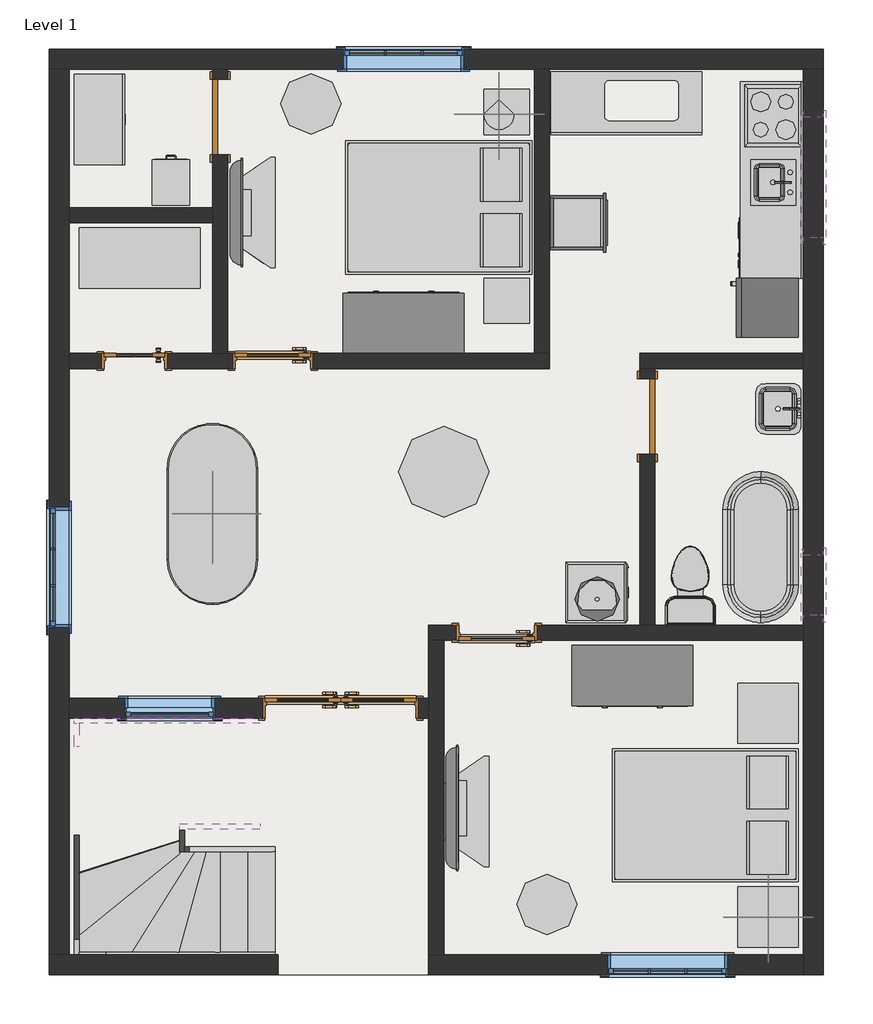
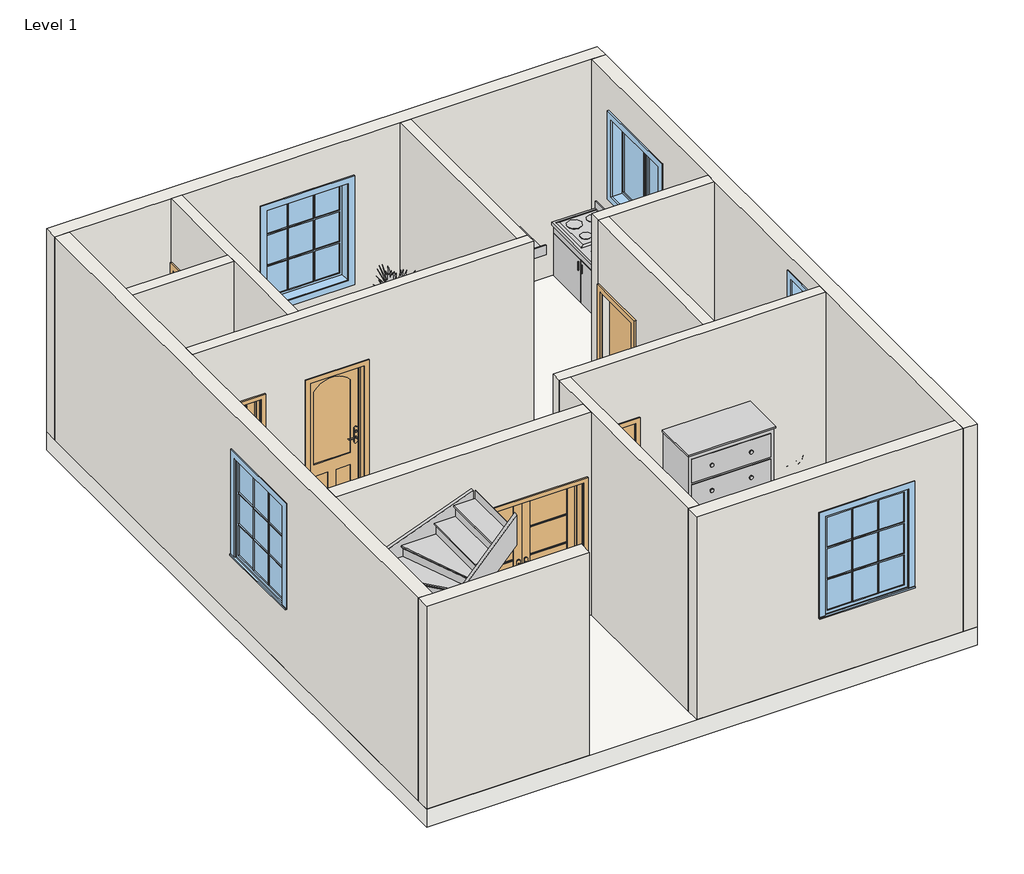
# One storey, incomplete: 22 furniture elements, 14 walls, 8 members, 6 doors, 6 windows, 5 flow terminals, 5 proxies, 3 geographic elements, 2 other elements.
"""IFC4 building model written with IfcOpenShell, lengths in millimetres."""

from ifc_helpers import new_model, si_unit, frame, origin, origin_with_axes, place, context, project, spatial, polyline, outline, extrude, faceted_brep, transform, mapped, element, save
from components import proxy_a6faaae8, proxy_45b28599, kitchenette_medium_kitchenette_medium_844211aa, proxy_8b8c2dc4, proxy_c523a7b7, door_4b146b56, door_14b9be53, door_b03bd389, door_6d64ae12, door_255cab33, door_059fdd7e, flow_terminal_871c2e40, flow_terminal_d49f872f, flow_terminal_62a433f7, toilet_domestic_3d_toilet_domestic_3d_f7549cf7, toilet_domestic_3d_toilet_domestic_3d_183bbd19, flow_terminal_b374fae2, furniture_6a014568, furniture_c8abb964, furniture_552c1472, furniture_c6510c7c, furniture_c9930e7d, furniture_2babcf72, furniture_9fa109b2, furniture_e1dba61b, furniture_7a3aaa4f, furniture_fdf74506, tv_stand_tv_stand_6ce107e5, furniture_2c34a4f9, furniture_905aceb5, furniture_f0d1c541, furniture_097b63cf, furniture_5bc9ed15, furniture_51091a24, rpc_plant_tropical_55f6ff97, rpc_plant_tropical_agave_1_5_93a2a214, stair_flight_22c751ce, window_cfa1ffdd, window_0862ab64, window_31198920, window_e41d21a6

model = new_model("IFC4")

# Units and contexts
model_context = context("Model", 3, world=origin())
ifc_project = project(units=[si_unit("LENGTHUNIT", "METRE", prefix="MILLI")], contexts=[model_context])

# Site, building, storey
site = spatial("IfcSite", under=ifc_project)
building = spatial("IfcBuilding", under=site)
storey = spatial("IfcBuildingStorey", under=building, Name="Level 1", Elevation=0.0)

# Proxies
placement = place(None, origin())
proxy_shape = proxy_a6faaae8(model_context)
element("IfcBuildingElementProxy", 1, Name="Cook Top-4 Unit2 : 22\" x 20\"", ObjectType="Cook Top-4 Unit2 : 22\" x 20\"", at=placement, inside=storey, context=model_context, shape_type="MappedRepresentation", body=[
    mapped(proxy_shape, transform((-2789.082173, 12884.8549175, 0.0), x_axis=(0.0, -1.0000000000000002, 0.0), y_axis=(1.0000000000000002, 0.0, 0.0), z_axis=(0.0, 0.0, 1.0))),
])
proxy_2_shape = proxy_45b28599(model_context)
element("IfcBuildingElementProxy", 2, Name="Dishwasher : 24\" x 24\" x 34\"", ObjectType="Dishwasher : 24\" x 24\" x 34\"", at=placement, inside=storey, context=model_context, shape_type="MappedRepresentation", body=[
    mapped(proxy_2_shape, transform((-3080.9317378, 11933.672386, 0.0), x_axis=(0.0, -1.0000000000000002, 0.0), y_axis=(1.0000000000000002, 0.0, 0.0), z_axis=(0.0, 0.0, 1.0))),
])
kitchenette_medium_kitchenette_medium_shape = kitchenette_medium_kitchenette_medium_844211aa(model_context)
element("IfcBuildingElementProxy", 3, Name="Kitchenette - Medium : Kitchenette - Medium", ObjectType="Kitchenette - Medium : Kitchenette - Medium", at=placement, inside=storey, context=model_context, shape_type="MappedRepresentation", body=[
    mapped(kitchenette_medium_kitchenette_medium_shape, transform((-2484.282173, 12560.6926225, 0.0), x_axis=(0.0, -1.0000000000000002, 0.0), y_axis=(1.0000000000000002, 0.0, 0.0), z_axis=(0.0, 0.0, 1.0))),
])
proxy_3_shape = proxy_8b8c2dc4(model_context)
element("IfcBuildingElementProxy", 4, Name="Oven Double-Built-in : 21 1/2\" x 39 1/4\" x 21\"", ObjectType="Oven Double-Built-in : 21 1/2\" x 39 1/4\" x 21\"", at=placement, inside=storey, context=model_context, shape_type="MappedRepresentation", body=[
    mapped(proxy_3_shape, transform((-4629.2163141, 11840.5298448, 0.0), x_axis=(0.0, 1.0000000000000009, 0.0), y_axis=(-1.0000000000000009, 0.0, 0.0), z_axis=(0.0, 0.0, 1.0))),
])
proxy_4_shape = proxy_c523a7b7(model_context)
element("IfcBuildingElementProxy", 5, Name="Refrigerator : 24\" x 25\" LH", ObjectType="Refrigerator : 24\" x 25\" LH", at=placement, inside=storey, context=model_context, shape_type="MappedRepresentation", body=[
    mapped(proxy_4_shape, transform((-2834.7311445, 10948.1049175, 0.0), x_axis=(0.0, -1.0000000000000002, 0.0), y_axis=(1.0000000000000002, 0.0, 0.0), z_axis=(0.0, 0.0, 1.0))),
])

# Doors
door_shape = door_4b146b56(model_context)
element("IfcDoor", 6, ObjectType="30\" x 80\"", at=placement, inside=storey, context=model_context, shape_type="MappedRepresentation", body=[
    mapped(door_shape, transform((-5583.082173, 7661.9799175, 0.0), x_axis=(1.0, 0.0, 0.0), y_axis=(0.0, 1.0, 0.0), z_axis=(0.0, 0.0, 1.0))),
])
door_2_shape = door_14b9be53(model_context)
element("IfcDoor", 7, ObjectType="30\" x 80\"", at=placement, inside=storey, context=model_context, shape_type="MappedRepresentation", body=[
    mapped(door_2_shape, transform((-7843.682173, 10411.5299175, 0.0), x_axis=(1.0, 0.0, 0.0), y_axis=(0.0, 1.0, 0.0), z_axis=(0.0, 0.0, 1.0))),
])
door_3_shape = door_b03bd389(model_context)
element("IfcDoor", 8, ObjectType="Door-Exterior-Double-Full Glass-Wood_Clad : 60\" x 80\"", at=placement, inside=storey, context=model_context, shape_type="MappedRepresentation", body=[
    mapped(door_3_shape, transform((-7157.882173, 6906.3299175, 0.0), x_axis=(1.0, 0.0, 0.0), y_axis=(0.0, 1.0, 0.0), z_axis=(0.0, 0.0, 1.0))),
])
door_4_shape = door_6d64ae12(model_context)
element("IfcDoor", 9, ObjectType="Door-Interior-Single-Full Glass-Wood : 24\" x 80\"", at=placement, inside=storey, context=model_context, shape_type="MappedRepresentation", body=[
    mapped(door_4_shape, transform((-9240.682173, 10411.5299175, 0.0), x_axis=(-1.0, 0.0, 0.0), y_axis=(0.0, -1.0, 0.0), z_axis=(0.0, 0.0, 1.0))),
])
door_5_shape = door_255cab33(model_context)
element("IfcDoor", 10, ObjectType="Single-Flush : 30\" x 80\"", at=placement, inside=storey, context=model_context, shape_type="MappedRepresentation", body=[
    mapped(door_5_shape, transform((-4059.082173, 9849.5549175, 0.0), x_axis=(0.0, 1.0, 0.0), y_axis=(-1.0, 0.0, 0.0), z_axis=(0.0, 0.0, 1.0))),
])
door_6_shape = door_059fdd7e(model_context)
element("IfcDoor", 11, ObjectType="Single-Flush : 30\" x 80\"", at=placement, inside=storey, context=model_context, shape_type="MappedRepresentation", body=[
    mapped(door_6_shape, transform((-8377.082173, 12872.1549175, 0.0), x_axis=(0.0, 1.0, 0.0), y_axis=(-1.0, 0.0, 0.0), z_axis=(0.0, 0.0, 1.0))),
])

# Flow terminals
flow_terminal_shape = flow_terminal_871c2e40(model_context)
element("IfcFlowTerminal", 12, ObjectType="Sink Kitchen-Island : 18\" x 18\"", at=placement, inside=storey, context=model_context, shape_type="MappedRepresentation", body=[
    mapped(flow_terminal_shape, transform((-2791.4275741, 12227.4441581, -14.4), x_axis=(0.0, -1.0000000000000002, 0.0), y_axis=(1.0000000000000002, 0.0, 0.0), z_axis=(0.0, 0.0, 1.0))),
])
flow_terminal_2_shape = flow_terminal_d49f872f(model_context)
element("IfcFlowTerminal", 13, ObjectType="Sink Vanity-Round : 19\" x 19\"", at=placement, inside=storey, context=model_context, shape_type="MappedRepresentation", body=[
    mapped(flow_terminal_2_shape, transform((-4470.4304324, 8089.8607114, 457.2), x_axis=(-1.0, 0.0, 0.0), y_axis=(0.0, -1.0, 0.0), z_axis=(0.0, 0.0, 1.0))),
])
flow_terminal_3_shape = flow_terminal_62a433f7(model_context)
element("IfcFlowTerminal", 14, ObjectType="Sink Vanity-Square : 20\" x 18\"", at=placement, inside=storey, context=model_context, shape_type="MappedRepresentation", body=[
    mapped(flow_terminal_3_shape, transform((-2689.8275741, 9941.4441581, 0.0), x_axis=(0.0, -1.0000000000000004, 0.0), y_axis=(1.0000000000000004, 0.0, 0.0), z_axis=(0.0, 0.0, 1.0))),
])
toilet_domestic_3d_toilet_domestic_3d_shape = toilet_domestic_3d_toilet_domestic_3d_f7549cf7(model_context)
toilet_domestic_3d_toilet_domestic_3d_2_shape = toilet_domestic_3d_toilet_domestic_3d_183bbd19(model_context)
element("IfcFlowTerminal", 15, ObjectType="Toilet-Domestic-3D : Toilet-Domestic-3D", at=placement, inside=storey, context=model_context, shape_type="MappedRepresentation", body=[
    mapped(toilet_domestic_3d_toilet_domestic_3d_shape, transform((-3627.282173, 8236.0509449, 0.0), x_axis=(-1.0000000000000004, 0.0, 0.0), y_axis=(0.0, -1.0000000000000004, 0.0), z_axis=(0.0, 0.0, 1.0))),
    mapped(toilet_domestic_3d_toilet_domestic_3d_2_shape, transform((-3627.282173, 8236.0509449, 0.0), x_axis=(-1.0000000000000004, 0.0, 0.0), y_axis=(0.0, -1.0000000000000004, 0.0), z_axis=(0.0, 0.0, 1.0))),
])
flow_terminal_4_shape = flow_terminal_b374fae2(model_context)
element("IfcFlowTerminal", 16, ObjectType="Tub-Free Standing-3D : 30\" x 60\"", at=placement, inside=storey, context=model_context, shape_type="MappedRepresentation", body=[
    mapped(flow_terminal_4_shape, transform((-2916.082173, 8528.7549175, 0.0), x_axis=(-1.0000000000000004, 0.0, 0.0), y_axis=(0.0, -1.0000000000000004, 0.0), z_axis=(0.0, 0.0, 1.0))),
])

# Furniture
furniture_shape = furniture_6a014568(model_context)
element("IfcFurniture", 17, ObjectType="24\"", at=placement, inside=storey, context=model_context, shape_type="MappedRepresentation", body=[
    mapped(furniture_shape, transform((-4884.582173, 8052.8172126, 0.0), x_axis=(0.0, 1.0, 0.0), y_axis=(-1.0, 0.0, 0.0), z_axis=(0.0, 0.0, 1.0))),
])
furniture_2_shape = furniture_c8abb964(model_context)
element("IfcFurniture", 18, ObjectType="Bed-Box : Double 53\" x 74\"", at=placement, inside=storey, context=model_context, shape_type="MappedRepresentation", body=[
    mapped(furniture_2_shape, transform((-3240.4526648, 6162.8073766, 0.0), x_axis=(0.0, -0.9999999999999998, 0.0), y_axis=(0.9999999999999998, 0.0, 0.0), z_axis=(0.0, 0.0, 1.0))),
])
element("IfcFurniture", 19, ObjectType="Bed-Box : Double 53\" x 74\"", at=placement, inside=storey, context=model_context, shape_type="MappedRepresentation", body=[
    mapped(furniture_2_shape, transform((-5932.8526648, 12296.9073766, 0.0), x_axis=(0.0, -1.0000000000000002, 0.0), y_axis=(1.0000000000000002, 0.0, 0.0), z_axis=(0.0, 0.0, 1.0))),
])
furniture_3_shape = furniture_552c1472(model_context)
element("IfcFurniture", 20, ObjectType="Cabinet-File 3 Drawer.0001 : 15\" x 18\"", at=placement, inside=storey, context=model_context, shape_type="MappedRepresentation", body=[
    mapped(furniture_3_shape, transform((-9000.27862, 12069.6206174, 0.0), x_axis=(-1.0000000000000004, 0.0, 0.0), y_axis=(0.0, -1.0000000000000004, 0.0), z_axis=(0.0, 0.0, 1.0))),
])
furniture_4_shape = furniture_c6510c7c(model_context)
element("IfcFurniture", 21, ObjectType="Counter Top w Sink Hole : 24\" Depth", at=placement, inside=storey, context=model_context, shape_type="MappedRepresentation", body=[
    mapped(furniture_4_shape, transform((-2484.282173, 12027.2926225, -14.4), x_axis=(0.0, -1.0000000000000002, 0.0), y_axis=(1.0000000000000002, 0.0, 0.0), z_axis=(0.0, 0.0, 1.0))),
])
furniture_5_shape = furniture_c9930e7d(model_context)
element("IfcFurniture", 22, ObjectType="Counter Top w Sink Hole : 24\" Depth", at=placement, inside=storey, context=model_context, shape_type="MappedRepresentation", body=[
    mapped(furniture_5_shape, transform((-4708.7182214, 12694.3549175, 0.0), x_axis=(-1.0, 0.0, 0.0), y_axis=(0.0, -1.0, 0.0), z_axis=(0.0, 0.0, 1.0))),
])
furniture_6_shape = furniture_2babcf72(model_context)
element("IfcFurniture", 23, ObjectType="Dresser : 48\" x 60\" x 24\"", at=placement, inside=storey, context=model_context, shape_type="MappedRepresentation", body=[
    mapped(furniture_6_shape, transform((-6792.0754328, 10426.1919634, 0.0), x_axis=(-1.0000000000000004, 0.0, 0.0), y_axis=(0.0, -1.0000000000000004, 0.0), z_axis=(0.0, 0.0, 1.0))),
])
furniture_7_shape = furniture_9fa109b2(model_context)
element("IfcFurniture", 24, ObjectType="Dresser : 48\" x 72\" x 24\"", at=placement, inside=storey, context=model_context, shape_type="MappedRepresentation", body=[
    mapped(furniture_7_shape, transform((-3941.830498, 7596.5178716, 0.0), x_axis=(1.0, 0.0, 0.0), y_axis=(0.0, 1.0, 0.0), z_axis=(0.0, 0.0, 1.0))),
])
furniture_8_shape = furniture_e1dba61b(model_context)
element("IfcFurniture", 25, ObjectType="Storage Pedestal : 20\" x 36\" x 36\"", at=placement, inside=storey, context=model_context, shape_type="MappedRepresentation", body=[
    mapped(furniture_8_shape, transform((-10530.6005491, 13026.7774315, 0.0), x_axis=(0.0, 1.000000000000001, 0.0), y_axis=(-1.000000000000001, 0.0, 0.0), z_axis=(0.0, 0.0, 1.0))),
])
furniture_9_shape = furniture_7a3aaa4f(model_context)
element("IfcFurniture", 26, ObjectType="TV - Flat Screen : 42\"", at=placement, inside=storey, context=model_context, shape_type="MappedRepresentation", body=[
    mapped(furniture_9_shape, transform((-8216.9435494, 11910.8994317, 914.4), x_axis=(0.0, 1.0000000000000002, 0.0), y_axis=(-1.0000000000000002, 0.0, 0.0), z_axis=(0.0, 0.0, 1.0))),
])
furniture_10_shape = furniture_fdf74506(model_context)
element("IfcFurniture", 27, ObjectType="TV - Flat Screen : 50\"", at=placement, inside=storey, context=model_context, shape_type="MappedRepresentation", body=[
    mapped(furniture_10_shape, transform((-6037.9435494, 5898.1815114, 914.4), x_axis=(0.0, 1.0, 0.0), y_axis=(-1.0, 0.0, 0.0), z_axis=(0.0, 0.0, 1.0))),
])
tv_stand_tv_stand_shape = tv_stand_tv_stand_6ce107e5(model_context)
element("IfcFurniture", 28, ObjectType="TV Stand : TV Stand", at=placement, inside=storey, context=model_context, shape_type="MappedRepresentation", body=[
    mapped(tv_stand_tv_stand_shape, transform((-6116.482173, 5736.5669155, 0.0), x_axis=(0.0, 1.0000000000000002, 0.0), y_axis=(-1.0000000000000002, 0.0, 0.0), z_axis=(0.0, 0.0, 1.0))),
])
element("IfcFurniture", 29, ObjectType="TV Stand : TV Stand", at=placement, inside=storey, context=model_context, shape_type="MappedRepresentation", body=[
    mapped(tv_stand_tv_stand_shape, transform((-8275.482173, 11781.7669155, 0.0), x_axis=(0.0, 1.0000000000000002, 0.0), y_axis=(-1.0000000000000002, 0.0, 0.0), z_axis=(0.0, 0.0, 1.0))),
])
furniture_11_shape = furniture_2c34a4f9(model_context)
element("IfcFurniture", 30, ObjectType="Table-Dining Oval : 36\" x 72\"", at=placement, inside=storey, context=model_context, shape_type="MappedRepresentation", body=[
    mapped(furniture_11_shape, transform((-8811.3805337, 9266.7122138, 0.0), x_axis=(0.0, 1.0, 0.0), y_axis=(-1.0, 0.0, 0.0), z_axis=(0.0, 0.0, 1.0))),
])
furniture_12_shape = furniture_905aceb5(model_context)
element("IfcFurniture", 31, ObjectType="Table-Dining Round w Chairs : 36\" Diameter", at=placement, inside=storey, context=model_context, shape_type="MappedRepresentation", body=[
    mapped(furniture_12_shape, transform((-6220.1641402, 9475.6336061, 0.0), x_axis=(1.0, 0.0, 0.0), y_axis=(0.0, 1.0, 0.0), z_axis=(0.0, 0.0, 1.0))),
])
furniture_13_shape = furniture_f0d1c541(model_context)
element("IfcFurniture", 32, ObjectType="Table-Ellipse : 72\" x 36\"", at=placement, inside=storey, context=model_context, shape_type="MappedRepresentation", body=[
    mapped(furniture_13_shape, transform((-5075.082173, 4921.9549175, 0.0), x_axis=(-1.0000000000000004, 0.0, 0.0), y_axis=(0.0, -1.0000000000000004, 0.0), z_axis=(0.0, 0.0, 1.0))),
])
element("IfcFurniture", 33, ObjectType="Table-Ellipse : 72\" x 36\"", at=placement, inside=storey, context=model_context, shape_type="MappedRepresentation", body=[
    mapped(furniture_13_shape, transform((-7459.1574537, 13005.1582156, 0.0), x_axis=(0.0, 1.000000000000001, 0.0), y_axis=(-1.000000000000001, 0.0, 0.0), z_axis=(0.0, 0.0, 1.0))),
])
furniture_14_shape = furniture_097b63cf(model_context)
element("IfcFurniture", 34, ObjectType="Table-Night Stand : 18\" x 18\" x 24\"", at=placement, inside=storey, context=model_context, shape_type="MappedRepresentation", body=[
    mapped(furniture_14_shape, transform((-5713.8158033, 10789.3549175, 0.0), x_axis=(1.0, 0.0, 0.0), y_axis=(0.0, 1.0, 0.0), z_axis=(0.0, 0.0, 1.0))),
])
element("IfcFurniture", 35, ObjectType="Table-Night Stand : 18\" x 18\" x 24\"", at=placement, inside=storey, context=model_context, shape_type="MappedRepresentation", body=[
    mapped(furniture_14_shape, transform((-5713.8158033, 12694.3549175, 0.0), x_axis=(1.0, 0.0, 0.0), y_axis=(0.0, 1.0, 0.0), z_axis=(0.0, 0.0, 1.0))),
])
furniture_15_shape = furniture_5bc9ed15(model_context)
element("IfcFurniture", 36, ObjectType="Table-Night Stand : 24\" x 24\" x 30\"", at=placement, inside=storey, context=model_context, shape_type="MappedRepresentation", body=[
    mapped(furniture_15_shape, transform((-3148.4158033, 4490.1549175, 0.0), x_axis=(1.0, 0.0, 0.0), y_axis=(0.0, 1.0, 0.0), z_axis=(0.0, 0.0, 1.0))),
])
element("IfcFurniture", 37, ObjectType="Table-Night Stand : 24\" x 24\" x 30\"", at=placement, inside=storey, context=model_context, shape_type="MappedRepresentation", body=[
    mapped(furniture_15_shape, transform((-3148.4158033, 6547.5549175, 0.0), x_axis=(1.0, 0.0, 0.0), y_axis=(0.0, 1.0, 0.0), z_axis=(0.0, 0.0, 1.0))),
])
furniture_16_shape = furniture_51091a24(model_context)
element("IfcFurniture", 38, ObjectType="Table-Rectangular : 72\" x 30\"", at=placement, inside=storey, context=model_context, shape_type="MappedRepresentation", body=[
    mapped(furniture_16_shape, transform((-9189.882173, 11449.7549175, 0.0), x_axis=(1.0, 0.0, 0.0), y_axis=(0.0, 1.0, 0.0), z_axis=(0.0, 0.0, 1.0))),
])

# Geographic elements
rpc_plant_tropical_shape = rpc_plant_tropical_55f6ff97(model_context)
element("IfcGeographicElement", 39, ObjectType="RPC Plant - Tropical", at=placement, inside=storey, context=model_context, shape_type="MappedRepresentation", body=[
    mapped(rpc_plant_tropical_shape, transform((-8453.282173, 8864.8925416, 609.6), x_axis=(1.0, 0.0, 0.0), y_axis=(0.0, 1.0, 0.0), z_axis=(0.0, 0.0, 1.0))),
])
rpc_plant_tropical_agave_1_5_shape = rpc_plant_tropical_agave_1_5_93a2a214(model_context)
element("IfcGeographicElement", 40, ObjectType="RPC Plant - Tropical : Agave - 1.5'", at=placement, inside=storey, context=model_context, shape_type="MappedRepresentation", body=[
    mapped(rpc_plant_tropical_agave_1_5_shape, transform((-5557.682173, 12897.5549175, 762.0), x_axis=(1.0, 0.0, 0.0), y_axis=(0.0, 1.0, 0.0), z_axis=(0.0, 0.0, 1.0))),
])
element("IfcGeographicElement", 41, ObjectType="RPC Plant - Tropical : Agave - 1.5'", at=placement, inside=storey, context=model_context, shape_type="MappedRepresentation", body=[
    mapped(rpc_plant_tropical_agave_1_5_shape, transform((-2839.882173, 4794.9549175, 762.0), x_axis=(1.0, 0.0, 0.0), y_axis=(0.0, 1.0, 0.0), z_axis=(0.0, 0.0, 1.0))),
])

# Members
element("IfcMember", 42, ObjectType="Stringer - 2\" Width", at=placement, inside=storey, context=model_context, shape_type="SweptSolid", body=[
    extrude(outline(polyline([(83.5564967, -7818.2848745), (415.8418245, -7818.2848745), (1159.7595923, -9531.8106114), (827.4742644, -9531.8106114), (83.5564967, -7818.2848745)])), frame((0.0, 4388.5549175, 0.0), z_axis=(0.0, 1.0, 0.0), x_axis=(0.0, 0.0, 1.0)), (0.0, 0.0, 1.0), 50.8),
])
element("IfcMember", 43, ObjectType="Stringer - 2\" Width", at=placement, inside=storey, context=model_context, shape_type="SweptSolid", body=[
    extrude(outline(polyline([(-9531.8106114, 4439.3549175), (-9531.8106114, 4388.5549175), (-9799.482173, 4388.5549175), (-9799.482173, 4439.3549175), (-9531.8106114, 4439.3549175)])), frame((0.0, 0.0, 827.4742644), z_axis=(0.0, 0.0, 1.0), x_axis=(1.0, 0.0, 0.0)), (0.0, 0.0, 1.0), 332.2853278),
])
element("IfcMember", 44, ObjectType="Stringer - 2\" Width", at=placement, inside=storey, context=model_context, shape_type="SweptSolid", body=[
    extrude(outline(polyline([(4388.5549175, 854.9595923), (4388.5549175, 1143.7120466), (6514.0452981, 1815.1471627), (6514.0452981, 1482.8618349), (4526.3622821, 854.9595923), (4388.5549175, 854.9595923)])), frame((-9850.282173, 0.0, 0.0), z_axis=(1.0, 0.0, 0.0), x_axis=(0.0, 1.0, 0.0)), (0.0, 0.0, 1.0), 50.8),
])
element("IfcMember", 45, ObjectType="Stringer - 2\" Width", at=placement, inside=storey, context=model_context, shape_type="SweptSolid", body=[
    extrude(outline(polyline([(-9799.482173, 6514.0452981), (-9850.282173, 6514.0452981), (-9850.282173, 6750.7549175), (-9799.482173, 6750.7549175), (-9799.482173, 6514.0452981)])), frame((0.0, 0.0, 1489.2492928), z_axis=(0.0, 0.0, 1.0), x_axis=(1.0, 0.0, 0.0)), (0.0, 0.0, 1.0), 319.6465141),
])
element("IfcMember", 46, ObjectType="Stringer - 2\" Width", at=placement, inside=storey, context=model_context, shape_type="SweptSolid", body=[
    extrude(outline(polyline([(1789.6968643, -9850.282173), (1504.0958069, -9850.282173), (1504.0958069, -9760.1986078), (2179.5047781, -7973.0806206), (2499.1512922, -7973.0806206), (1789.6968643, -9850.282173)])), frame((0.0, 6750.7549175, 0.0), z_axis=(0.0, 1.0, 0.0), x_axis=(0.0, 0.0, 1.0)), (0.0, 0.0, 1.0), 50.8),
])
element("IfcMember", 47, ObjectType="Stringer - 2\" Width", at=placement, inside=storey, context=model_context, shape_type="SweptSolid", body=[
    extrude(outline(polyline([(0.0, -7818.2848745), (314.6605696, -7818.2848745), (1250.7228943, -8732.682173), (814.5341975, -8732.682173), (0.0, -7937.000251), (0.0, -7818.2848745)])), frame((0.0, 5455.3549175, 0.0), z_axis=(0.0, 1.0, 0.0), x_axis=(0.0, 0.0, 1.0)), (0.0, 0.0, 1.0), 50.8),
])
element("IfcMember", 48, ObjectType="Stringer - 2\" Width", at=placement, inside=storey, context=model_context, shape_type="SweptSolid", body=[
    extrude(outline(polyline([(5455.3549175, 866.5378136), (5455.3549175, 1470.7613416), (5640.3509671, 1890.0468689), (5683.9549175, 1890.0468689), (5683.9549175, 1233.8039522), (5521.9107248, 866.5378136), (5455.3549175, 866.5378136)])), frame((-8783.482173, 0.0, 0.0), z_axis=(1.0, 0.0, 0.0), x_axis=(0.0, 1.0, 0.0)), (0.0, 0.0, 1.0), 50.8),
])
element("IfcMember", 49, ObjectType="Stringer - 2\" Width", at=placement, inside=storey, context=model_context, shape_type="SweptSolid", body=[
    extrude(outline(polyline([(1890.0468689, -8783.482173), (1436.8245927, -8783.482173), (2328.6417632, -7973.0806206), (2781.8640394, -7973.0806206), (1890.0468689, -8783.482173)])), frame((0.0, 5683.9549175, 0.0), z_axis=(0.0, 1.0, 0.0), x_axis=(0.0, 0.0, 1.0)), (0.0, 0.0, 1.0), 50.8),
])

# Slab
element("IfcSlab", 50, ObjectType="Wood Joist 10\" - Ceramic Tile", at=placement, inside=storey, context=model_context, shape_type="SweptSolid", body=[
    extrude(outline(polyline([(-2281.082173, 13557.9549175), (-2281.082173, 4210.7549175), (-10104.282173, 4210.7549175), (-10104.282173, 13557.9549175), (-2281.082173, 13557.9549175)])), frame((0.0, 0.0, -273.05), z_axis=(0.0, 0.0, 1.0), x_axis=(1.0, 0.0, 0.0)), (0.0, 0.0, 1.0), 273.05),
])

# Stair flight
stair_flight_shape = stair_flight_22c751ce(model_context)
element("IfcStairFlight", 51, ObjectType="2\" Tread 1\" Nosing 1/4\" Riser", at=placement, inside=storey, context=model_context, shape_type="MappedRepresentation", body=[
    mapped(stair_flight_shape, transform((0.0, 0.0, 0.0), x_axis=(1.0, 0.0, 0.0), y_axis=(0.0, 1.0, 0.0), z_axis=(0.0, 0.0, 1.0))),
])

# Walls
element("IfcWall", 52, ObjectType="Generic - 8\"", at=placement, inside=storey, context=model_context, shape_type="Brep", body=[
    faceted_brep([(-10104.282173, 13354.7549175, 0.0), (-9901.082173, 13354.7549175, 0.0), (-8453.282173, 13354.7549175, 0.0), (-8300.882173, 13354.7549175, 0.0), (-5202.082173, 13354.7549175, 0.0), (-5049.682173, 13354.7549175, 0.0), (-2484.282173, 13354.7549175, 0.0), (-2281.082173, 13354.7549175, 0.0), (-2281.082173, 13354.7549175, 3048.0), (-2484.282173, 13354.7549175, 3048.0), (-5049.682173, 13354.7549175, 3048.0), (-5202.082173, 13354.7549175, 3048.0), (-8300.882173, 13354.7549175, 3048.0), (-8453.282173, 13354.7549175, 3048.0), (-9901.082173, 13354.7549175, 3048.0), (-10104.282173, 13354.7549175, 3048.0), (-5913.282173, 13354.7549175, 2438.4), (-5913.282173, 13354.7549175, 914.4), (-7132.482173, 13354.7549175, 914.4), (-7132.482173, 13354.7549175, 2438.4), (-10104.282173, 13557.9549175, 0.0), (-10104.282173, 13557.9549175, 3048.0), (-2281.082173, 13557.9549175, 3048.0), (-2281.082173, 13557.9549175, 0.0), (-5913.282173, 13557.9549175, 2438.4), (-7132.482173, 13557.9549175, 2438.4), (-7132.482173, 13557.9549175, 914.4), (-5913.282173, 13557.9549175, 914.4)], [[[0, 1, 2, 3, 4, 5, 6, 7, 8, 9, 10, 11, 12, 13, 14, 15], [16, 17, 18, 19]], [[20, 21, 22, 23], [24, 25, 26, 27]], [[7, 6, 5, 4, 3, 2, 1, 0, 20, 23]], [[8, 7, 23, 22]], [[0, 15, 21, 20]], [[15, 14, 13, 12, 11, 10, 9, 8, 22, 21]], [[17, 16, 24, 27]], [[18, 17, 27, 26]], [[19, 18, 26, 25]], [[16, 19, 25, 24]]]),
])
element("IfcWall", 53, ObjectType="Generic - 8\"", at=placement, inside=storey, context=model_context, shape_type="Brep", body=[
    faceted_brep([(-2484.282173, 13354.7549175, 0.0), (-2484.282173, 10484.5549175, 0.0), (-2484.282173, 10332.1549175, 0.0), (-2484.282173, 7741.3549175, 0.0), (-2484.282173, 7588.9549175, 0.0), (-2484.282173, 4413.9549175, 0.0), (-2484.282173, 4210.7549175, 0.0), (-2484.282173, 4210.7549175, 3048.0), (-2484.282173, 4413.9549175, 3048.0), (-2484.282173, 7588.9549175, 3048.0), (-2484.282173, 7741.3549175, 3048.0), (-2484.282173, 10332.1549175, 3048.0), (-2484.282173, 10484.5549175, 3048.0), (-2484.282173, 13354.7549175, 3048.0), (-2484.282173, 11652.9549175, 2489.2), (-2484.282173, 11652.9549175, 1270.0), (-2484.282173, 12872.1549175, 1270.0), (-2484.282173, 12872.1549175, 2489.2), (-2484.282173, 7842.9549175, 2768.6), (-2484.282173, 7842.9549175, 2159.0), (-2484.282173, 8452.5549175, 2159.0), (-2484.282173, 8452.5549175, 2768.6), (-2281.082173, 13354.7549175, 0.0), (-2281.082173, 13354.7549175, 3048.0), (-2281.082173, 4210.7549175, 3048.0), (-2281.082173, 4210.7549175, 0.0), (-2281.082173, 11652.9549175, 2489.2), (-2281.082173, 12872.1549175, 2489.2), (-2281.082173, 12872.1549175, 1270.0), (-2281.082173, 11652.9549175, 1270.0), (-2281.082173, 7842.9549175, 2768.6), (-2281.082173, 8452.5549175, 2768.6), (-2281.082173, 8452.5549175, 2159.0), (-2281.082173, 7842.9549175, 2159.0)], [[[0, 1, 2, 3, 4, 5, 6, 7, 8, 9, 10, 11, 12, 13], [14, 15, 16, 17], [18, 19, 20, 21]], [[22, 23, 24, 25], [26, 27, 28, 29], [30, 31, 32, 33]], [[6, 5, 4, 3, 2, 1, 0, 22, 25]], [[0, 13, 23, 22]], [[7, 6, 25, 24]], [[13, 12, 11, 10, 9, 8, 7, 24, 23]], [[15, 14, 26, 29]], [[16, 15, 29, 28]], [[17, 16, 28, 27]], [[14, 17, 27, 26]], [[19, 18, 30, 33]], [[20, 19, 33, 32]], [[21, 20, 32, 31]], [[18, 21, 31, 30]]]),
])
element("IfcWall", 54, ObjectType="Generic - 8\"", at=placement, inside=storey, context=model_context, shape_type="Brep", body=[
    faceted_brep([(-2484.282173, 4413.9549175, 0.0), (-6116.482173, 4413.9549175, 0.0), (-6268.882173, 4413.9549175, 0.0), (-6268.882173, 4413.9549175, 3048.0), (-6116.482173, 4413.9549175, 3048.0), (-2484.282173, 4413.9549175, 3048.0), (-4465.482173, 4413.9549175, 2438.4), (-4465.482173, 4413.9549175, 914.4), (-3246.282173, 4413.9549175, 914.4), (-3246.282173, 4413.9549175, 2438.4), (-2484.282173, 4210.7549175, 0.0), (-2484.282173, 4210.7549175, 3048.0), (-6268.882173, 4210.7549175, 3048.0), (-6268.882173, 4210.7549175, 0.0), (-4465.482173, 4210.7549175, 2438.4), (-3246.282173, 4210.7549175, 2438.4), (-3246.282173, 4210.7549175, 914.4), (-4465.482173, 4210.7549175, 914.4)], [[[0, 1, 2, 3, 4, 5], [6, 7, 8, 9]], [[10, 11, 12, 13], [14, 15, 16, 17]], [[2, 1, 0, 10, 13]], [[0, 5, 11, 10]], [[3, 2, 13, 12]], [[5, 4, 3, 12, 11]], [[7, 6, 14, 17]], [[8, 7, 17, 16]], [[9, 8, 16, 15]], [[6, 9, 15, 14]]]),
])
element("IfcWall", 55, ObjectType="Generic - 8\"", at=placement, inside=storey, context=model_context, shape_type="Brep", body=[
    faceted_brep([(-9901.082173, 4413.9549175, 0.0), (-9901.082173, 6801.5549175, 0.0), (-9901.082173, 7004.7549175, 0.0), (-9901.082173, 10332.1549175, 0.0), (-9901.082173, 10484.5549175, 0.0), (-9901.082173, 11805.3549175, 0.0), (-9901.082173, 11957.7549175, 0.0), (-9901.082173, 13354.7549175, 0.0), (-9901.082173, 13354.7549175, 3048.0), (-9901.082173, 11957.7549175, 3048.0), (-9901.082173, 11805.3549175, 3048.0), (-9901.082173, 10484.5549175, 3048.0), (-9901.082173, 10332.1549175, 3048.0), (-9901.082173, 7004.7549175, 3048.0), (-9901.082173, 6801.5549175, 3048.0), (-9901.082173, 4413.9549175, 3048.0), (-9901.082173, 8935.1549175, 2438.4), (-9901.082173, 8935.1549175, 914.4), (-9901.082173, 7715.9549175, 914.4), (-9901.082173, 7715.9549175, 2438.4), (-10104.282173, 4413.9549175, 0.0), (-10104.282173, 4413.9549175, 3048.0), (-10104.282173, 13354.7549175, 3048.0), (-10104.282173, 13354.7549175, 0.0), (-10104.282173, 8935.1549175, 2438.4), (-10104.282173, 7715.9549175, 2438.4), (-10104.282173, 7715.9549175, 914.4), (-10104.282173, 8935.1549175, 914.4)], [[[0, 1, 2, 3, 4, 5, 6, 7, 8, 9, 10, 11, 12, 13, 14, 15], [16, 17, 18, 19]], [[20, 21, 22, 23], [24, 25, 26, 27]], [[7, 6, 5, 4, 3, 2, 1, 0, 20, 23]], [[8, 7, 23, 22]], [[0, 15, 21, 20]], [[15, 14, 13, 12, 11, 10, 9, 8, 22, 21]], [[17, 16, 24, 27]], [[18, 17, 27, 26]], [[19, 18, 26, 25]], [[16, 19, 25, 24]]]),
])
element("IfcWall", 56, ObjectType="Generic - 8\"", at=placement, inside=storey, context=model_context, shape_type="SweptSolid", body=[
    extrude(outline(polyline([(3048.0, -9901.082173), (0.0, -9901.082173), (0.0, -7945.282173), (2057.4, -7945.282173), (2057.4, -6370.482173), (0.0, -6370.482173), (0.0, -6268.882173), (3048.0, -6268.882173), (3048.0, -9901.082173)]), holes=[polyline([(1778.0, -9342.282173), (1778.0, -8427.882173), (558.8, -8427.882173), (558.8, -9342.282173), (1778.0, -9342.282173)])]), frame((0.0, 6801.5549175, 0.0), z_axis=(0.0, 1.0, 0.0), x_axis=(0.0, 0.0, 1.0)), (0.0, 0.0, 1.0), 203.2),
])
element("IfcWall", 57, ObjectType="Generic - 8\"", at=placement, inside=storey, context=model_context, shape_type="Brep", body=[
    faceted_brep([(-7792.882173, 4413.9549175, 0.0), (-9901.082173, 4413.9549175, 0.0), (-10104.282173, 4413.9549175, 0.0), (-10104.282173, 4413.9549175, 3048.0), (-9901.082173, 4413.9549175, 3048.0), (-7792.882173, 4413.9549175, 3048.0), (-7792.882173, 4210.7549175, 0.0), (-7792.882173, 4210.7549175, 3048.0), (-10104.282173, 4210.7549175, 3048.0), (-10104.282173, 4210.7549175, 0.0)], [[[0, 1, 2, 3, 4, 5]], [[6, 7, 8, 9]], [[2, 1, 0, 6, 9]], [[0, 5, 7, 6]], [[3, 2, 9, 8]], [[5, 4, 3, 8, 7]]]),
])
element("IfcWall", 58, ObjectType="INNER WALL", at=placement, inside=storey, context=model_context, shape_type="Brep", body=[
    faceted_brep([(-2484.282173, 10484.5549175, 0.0), (-4135.282173, 10484.5549175, 0.0), (-4135.282173, 10484.5549175, 3048.0), (-2484.282173, 10484.5549175, 3048.0), (-2484.282173, 10332.1549175, 0.0), (-2484.282173, 10332.1549175, 3048.0), (-3982.882173, 10332.1549175, 3048.0), (-4135.282173, 10332.1549175, 3048.0), (-4135.282173, 10332.1549175, 0.0), (-3982.882173, 10332.1549175, 0.0)], [[[0, 1, 2, 3]], [[4, 5, 6, 7, 8, 9]], [[1, 0, 4, 9, 8]], [[0, 3, 5, 4]], [[2, 1, 8, 7]], [[3, 2, 7, 6, 5]]]),
])
element("IfcWall", 59, ObjectType="INNER WALL", at=placement, inside=storey, context=model_context, shape_type="SweptSolid", body=[
    extrude(outline(polyline([(-5202.082173, 10484.5549175), (-5202.082173, 13354.7549175), (-5049.682173, 13354.7549175), (-5049.682173, 10484.5549175), (-5202.082173, 10484.5549175)])), origin_with_axes(), (0.0, 0.0, 1.0), 3048.0),
])
element("IfcWall", 60, ObjectType="INNER WALL", at=placement, inside=storey, context=model_context, shape_type="Brep", body=[
    faceted_brep([(-8300.882173, 13253.1549175, 2032.0), (-8300.882173, 13253.1549175, 0.0), (-8300.882173, 13354.7549175, 0.0), (-8300.882173, 13354.7549175, 3048.0), (-8300.882173, 10484.5549175, 3048.0), (-8300.882173, 10484.5549175, 0.0), (-8300.882173, 12491.1549175, 0.0), (-8300.882173, 12491.1549175, 2032.0), (-8453.282173, 13354.7549175, 0.0), (-8453.282173, 13253.1549175, 0.0), (-8453.282173, 13253.1549175, 2032.0), (-8453.282173, 12491.1549175, 2032.0), (-8453.282173, 12491.1549175, 0.0), (-8453.282173, 11957.7549175, 0.0), (-8453.282173, 11805.3549175, 0.0), (-8453.282173, 10484.5549175, 0.0), (-8453.282173, 10484.5549175, 3048.0), (-8453.282173, 11805.3549175, 3048.0), (-8453.282173, 11957.7549175, 3048.0), (-8453.282173, 13354.7549175, 3048.0)], [[[0, 1, 2, 3, 4, 5, 6, 7]], [[8, 9, 10, 11, 12, 13, 14, 15, 16, 17, 18, 19]], [[6, 5, 15, 14, 13, 12]], [[2, 1, 9, 8]], [[3, 2, 8, 19]], [[5, 4, 16, 15]], [[10, 9, 1, 0]], [[11, 10, 0, 7]], [[12, 11, 7, 6]], [[4, 3, 19, 18, 17, 16]]]),
])
element("IfcWall", 61, ObjectType="INNER WALL", at=placement, inside=storey, context=model_context, shape_type="Brep", body=[
    faceted_brep([(-2484.282173, 7741.3549175, 3048.0), (-2484.282173, 7741.3549175, 0.0), (-3982.882173, 7741.3549175, 0.0), (-4135.282173, 7741.3549175, 0.0), (-5176.682173, 7741.3549175, 0.0), (-5176.682173, 7741.3549175, 2057.4), (-5989.482173, 7741.3549175, 2057.4), (-5989.482173, 7741.3549175, 0.0), (-6268.882173, 7741.3549175, 0.0), (-6268.882173, 7741.3549175, 3048.0), (-4135.282173, 7741.3549175, 3048.0), (-3982.882173, 7741.3549175, 3048.0), (-2484.282173, 7588.9549175, 0.0), (-2484.282173, 7588.9549175, 3048.0), (-6116.482173, 7588.9549175, 3048.0), (-6268.882173, 7588.9549175, 3048.0), (-6268.882173, 7588.9549175, 0.0), (-6116.482173, 7588.9549175, 0.0), (-5989.482173, 7588.9549175, 0.0), (-5989.482173, 7588.9549175, 2057.4), (-5176.682173, 7588.9549175, 2057.4), (-5176.682173, 7588.9549175, 0.0)], [[[0, 1, 2, 3, 4, 5, 6, 7, 8, 9, 10, 11]], [[12, 13, 14, 15, 16, 17, 18, 19, 20, 21]], [[1, 12, 21, 4, 3, 2]], [[16, 8, 7, 18, 17]], [[1, 0, 13, 12]], [[9, 8, 16, 15]], [[20, 5, 4, 21]], [[5, 20, 19, 6]], [[6, 19, 18, 7]], [[0, 11, 10, 9, 15, 14, 13]]]),
])
element("IfcWall", 62, ObjectType="INNER WALL", at=placement, inside=storey, context=model_context, shape_type="SweptSolid", body=[
    extrude(outline(polyline([(10332.1549175, 0.0), (10230.5549175, 0.0), (10230.5549175, 2032.0), (9468.5549175, 2032.0), (9468.5549175, 0.0), (7741.3549175, 0.0), (7741.3549175, 3048.0), (10332.1549175, 3048.0), (10332.1549175, 0.0)])), frame((-4135.282173, 0.0, 0.0), z_axis=(1.0, 0.0, 0.0), x_axis=(0.0, 1.0, 0.0)), (0.0, 0.0, 1.0), 152.4),
])
element("IfcWall", 63, ObjectType="INNER WALL", at=placement, inside=storey, context=model_context, shape_type="Brep", body=[
    faceted_brep([(-6268.882173, 7588.9549175, 0.0), (-6268.882173, 7004.7549175, 0.0), (-6268.882173, 6801.5549175, 0.0), (-6268.882173, 4413.9549175, 0.0), (-6268.882173, 4413.9549175, 3048.0), (-6268.882173, 6801.5549175, 3048.0), (-6268.882173, 7004.7549175, 3048.0), (-6268.882173, 7588.9549175, 3048.0), (-6116.482173, 7588.9549175, 0.0), (-6116.482173, 7588.9549175, 3048.0), (-6116.482173, 4413.9549175, 3048.0), (-6116.482173, 4413.9549175, 0.0)], [[[0, 1, 2, 3, 4, 5, 6, 7]], [[8, 9, 10, 11]], [[3, 2, 1, 0, 8, 11]], [[4, 3, 11, 10]], [[0, 7, 9, 8]], [[7, 6, 5, 4, 10, 9]]]),
])
element("IfcWall", 64, ObjectType="INNER WALL", at=placement, inside=storey, context=model_context, shape_type="SweptSolid", body=[
    extrude(outline(polyline([(-9901.082173, 11957.7549175), (-8453.282173, 11957.7549175), (-8453.282173, 11805.3549175), (-9901.082173, 11805.3549175), (-9901.082173, 11957.7549175)])), origin_with_axes(), (0.0, 0.0, 1.0), 3048.0),
])
element("IfcWall", 65, ObjectType="INNER WALL", at=placement, inside=storey, context=model_context, shape_type="Brep", body=[
    faceted_brep([(-5049.682173, 10484.5549175, 3048.0), (-5049.682173, 10484.5549175, 0.0), (-5202.082173, 10484.5549175, 0.0), (-7437.282173, 10484.5549175, 0.0), (-7437.282173, 10484.5549175, 2057.4), (-8250.082173, 10484.5549175, 2057.4), (-8250.082173, 10484.5549175, 0.0), (-8300.882173, 10484.5549175, 0.0), (-8453.282173, 10484.5549175, 0.0), (-8910.482173, 10484.5549175, 0.0), (-8910.482173, 10484.5549175, 2057.4), (-9570.882173, 10484.5549175, 2057.4), (-9570.882173, 10484.5549175, 0.0), (-9901.082173, 10484.5549175, 0.0), (-9901.082173, 10484.5549175, 3048.0), (-8453.282173, 10484.5549175, 3048.0), (-8300.882173, 10484.5549175, 3048.0), (-5202.082173, 10484.5549175, 3048.0), (-5049.682173, 10332.1549175, 0.0), (-5049.682173, 10332.1549175, 3048.0), (-9901.082173, 10332.1549175, 3048.0), (-9901.082173, 10332.1549175, 0.0), (-9570.882173, 10332.1549175, 0.0), (-9570.882173, 10332.1549175, 2057.4), (-8910.482173, 10332.1549175, 2057.4), (-8910.482173, 10332.1549175, 0.0), (-8250.082173, 10332.1549175, 0.0), (-8250.082173, 10332.1549175, 2057.4), (-7437.282173, 10332.1549175, 2057.4), (-7437.282173, 10332.1549175, 0.0)], [[[0, 1, 2, 3, 4, 5, 6, 7, 8, 9, 10, 11, 12, 13, 14, 15, 16, 17]], [[18, 19, 20, 21, 22, 23, 24, 25, 26, 27, 28, 29]], [[1, 18, 29, 3, 2]], [[21, 13, 12, 22]], [[6, 26, 25, 9, 8, 7]], [[1, 0, 19, 18]], [[14, 13, 21, 20]], [[28, 4, 3, 29]], [[4, 28, 27, 5]], [[5, 27, 26, 6]], [[11, 23, 22, 12]], [[23, 11, 10, 24]], [[24, 10, 9, 25]], [[0, 17, 16, 15, 14, 20, 19]]]),
])

# Windows
window_shape = window_cfa1ffdd(model_context)
element("IfcWindow", 66, ObjectType="Casement 3x3 with Trim : 48\" x 60\"", at=placement, inside=storey, context=model_context, shape_type="MappedRepresentation", body=[
    mapped(window_shape, transform((-3855.882173, 4312.3549175, 304.8), x_axis=(-1.0, 0.0, 0.0), y_axis=(0.0, -1.0, 0.0), z_axis=(0.0, 0.0, 1.0))),
])
element("IfcWindow", 67, ObjectType="Casement 3x3 with Trim : 48\" x 60\"", at=placement, inside=storey, context=model_context, shape_type="MappedRepresentation", body=[
    mapped(window_shape, transform((-10002.682173, 8325.5549175, 304.8), x_axis=(0.0, 1.0, 0.0), y_axis=(-1.0, 0.0, 0.0), z_axis=(0.0, 0.0, 1.0))),
])
element("IfcWindow", 68, ObjectType="Casement 3x3 with Trim : 48\" x 60\"", at=placement, inside=storey, context=model_context, shape_type="MappedRepresentation", body=[
    mapped(window_shape, transform((-6522.882173, 13456.3549175, 304.8), x_axis=(1.0, 0.0, 0.0), y_axis=(0.0, 1.0, 0.0), z_axis=(0.0, 0.0, 1.0))),
])
window_2_shape = window_0862ab64(model_context)
element("IfcWindow", 69, ObjectType="Casement Dbl with Trim : 48\" x 48\"", at=placement, inside=storey, context=model_context, shape_type="MappedRepresentation", body=[
    mapped(window_2_shape, transform((-2401.732173, 12262.5549175, 355.6), x_axis=(0.0, -1.0, 0.0), y_axis=(1.0, 0.0, 0.0), z_axis=(0.0, 0.0, 1.0))),
])
window_3_shape = window_31198920(model_context)
element("IfcWindow", 70, ObjectType="Double Hung with Trim : 36\" x 48\"", at=placement, inside=storey, context=model_context, shape_type="MappedRepresentation", body=[
    mapped(window_3_shape, transform((-8885.082173, 6903.1549175, -355.6), x_axis=(-1.0, 0.0, 0.0), y_axis=(0.0, -1.0, 0.0), z_axis=(0.0, 0.0, 1.0))),
])
window_4_shape = window_e41d21a6(model_context)
element("IfcWindow", 71, ObjectType="Transom with Trim : 24\" x 24\"", at=placement, inside=storey, context=model_context, shape_type="MappedRepresentation", body=[
    mapped(window_4_shape, transform((-2382.682173, 8109.6549175, 0.0), x_axis=(0.0, -1.0, 0.0), y_axis=(1.0, 0.0, 0.0), z_axis=(0.0, 0.0, 1.0))),
])

save(model, "model.ifc")

# Revit data of these elements
# Type "Cook Top-4 Unit2 : 22\" x 20\""
#   Depth = 1' - 8"
#   Width = 1' - 10"
#   Burner Material = Steel, Chrome Plated
#   Cooktop Material = Steel, Polished
#   Default Elevation = 0
#   Assembly Code = ""
# Type "Dishwasher : 24\" x 24\" x 34\""
#   Label = "DW"
#   Assembly Code = "E1090400"
#   Depth = 2' - 0"
#   Height = 2' - 10"
#   Width = 2' - 0"
#   Dishwasher Material = Steel, Paint Finish, Ivory, Glossy
#   Panel Face Material = Plastic, Opaque Black
#   Default Elevation = 0
# Type "Kitchenette - Medium : Kitchenette - Medium"
#   Assembly Code = "E1090400"
#   Counter Length = 6' - 6"
#   Cabinet Width = 4' - 6"
#   Cabinet Height = 2' - 10 1/2"
#   Cabinet Depth = 2' - 0"
#   Toe Depth = 0' - 3"
#   Toe Height = 0' - 3 1/2"
#   Cabinet Material = Cabinets
#   Door/Drawer Material = Cabinets
#   Handle Material = Cabinets - Handles
#   Default Elevation = 0
# Type "Oven Double-Built-in : 21 1/2\" x 39 1/4\" x 21\""
#   Label = "OVEN"
#   Assembly Code = "E1090400"
#   Depth = 1' - 9"
#   Height = 3' - 3 1/4"
#   Width = 1' - 9 1/2"
#   Oven Material = Metal - Stainless Steel, Polished
#   Default Elevation = 0
# Type "Refrigerator : 24\" x 25\" LH"
#   Label = "REF."
#   Assembly Code = "E1090400"
#   Depth = 2' - 0 3/4"
#   Handle = 0' - 1 1/2"
#   Height = 5' - 3 1/2"
#   Rear Clearance = 0' - 2"
#   Top Door Height = 1' - 8"
#   Width = 1' - 11 1/2"
#   Material = Steel, Paint Finish, Ivory, Glossy
#   Default Elevation = 0
# Type "30\" x 80\""
#   Type Mark = "9"
#   Assembly Code = "B2030100"
#   Analytic Construction = "French door, wood frame with single glass"
#   Threshold Offset [instance default] = 0' - 0 1/2"
#   Thickness = 0' - 1 3/8"
#   Thermal Resistance (R) = 1.0696 (h·ft²·°F)/BTU
#   Swing Angle [instance default] = 90.00°
#   Stiles = 0' - 4 3/4"
#   Rough Width = 2' - 8"
#   Rough Height = 6' - 9"
#   Radius = 1' - 1.00625"
#   Lock Rail = 0' - 7 1/8"
#   Height = 6' - 8"
#   Width = 2' - 6"
#   Heat Transfer Coefficient (U) = 0.9350 BTU/(h·ft²·°F)
#   Door Offset [instance default] = 0' - 0"
#   Bottom Rail = 0' - 9 1/2"
#   Threshold [instance default] = yes
#   Function = 1
#   Exterior Trim [instance default] = yes
#   Trim Material = Cherry
#   Threshold Material = Cherry
#   Panel Material = Cherry
#   Glazing = Glass
#   Frame Material = Cherry
#   Door Handle Material = Aluminum
#   Visual Light Transmittance = 0
#   Solar Heat Gain Coefficient = 0
#   Wall Closure = (empty or 0)
#   Construction Type = (empty or 0)
# Type "Door-Exterior-Double-Full Glass-Wood_Clad : 60\" x 80\""
#   Type Mark = "8"
#   Assembly Code = "B2030100"
#   Analytic Construction = "French door, wood frame with double glass"
#   Top Rail = 0' - 4 11/16"
#   Threshold Offset [instance default] = 0' - 0 1/2"
#   Thickness = 0' - 1 3/8"
#   Thermal Resistance (R) = 1.9158 (h·ft²·°F)/BTU
#   Swing Angle [instance default] = 90.00°
#   Stiles = 0' - 4 3/4"
#   Rough Width = 5' - 2"
#   Rough Height = 6' - 9"
#   Panel Width = 2' - 6"
#   Door Offset [instance default] = 0' - 0"
#   Height = 6' - 8"
#   Width = 5' - 0"
#   Heat Transfer Coefficient (U) = 0.5220 BTU/(h·ft²·°F)
#   Bottom Rail = 0' - 9 1/8"
#   Exterior Trim [instance default] = yes
#   Threshold [instance default] = yes
#   Show Grill [instance default] = yes
#   Function = 1
#   Trim Material = Cherry
#   Threshold Material = Cherry
#   Panel Material = Cherry
#   Glazing = Glass
#   Frame Material = Cherry
#   Door Handle Material = Aluminum
#   Visual Light Transmittance = 0
#   Solar Heat Gain Coefficient = 0
#   Wall Closure = (empty or 0)
#   Construction Type = (empty or 0)
# Type "Door-Interior-Single-Full Glass-Wood : 24\" x 80\""
#   Type Mark = "10"
#   Assembly Code = "C1020300"
#   Analytic Construction = "Wood frame with single clear glass"
#   Top Rail = 0' - 4 11/16"
#   Thickness = 0' - 1 3/8"
#   Thermal Resistance (R) = 1.0102 (h·ft²·°F)/BTU
#   Swing Angle [instance default] = 90.00°
#   Stiles = 0' - 4 3/4"
#   Rough Width = 2' - 2"
#   Rough Height = 6' - 9"
#   Height = 6' - 8"
#   Width = 2' - 0"
#   Heat Transfer Coefficient (U) = 0.9900 BTU/(h·ft²·°F)
#   Bottom Rail = 0' - 9 1/8"
#   Show Grill [instance default] = yes
#   Trim Material = Cherry
#   Panel Material = Cherry
#   Frame Material = Cherry
#   Door Handle Material = Aluminum
#   Visual Light Transmittance = 0
#   Solar Heat Gain Coefficient = 0
#   Wall Closure = (empty or 0)
#   Function = (empty or 0)
# Type "Single-Flush : 30\" x 80\""
#   Type Mark = "5"
#   Construction Type Id = "MDOOR"
#   Assembly Code = "C1020"
#   Analytic Construction = "Metal"
#   Thickness = 0' - 2"
#   Heat Transfer Coefficient (U) = 0.651978 BTU/(h·ft²·°F)
#   Height = 6' - 8"
#   Trim Projection Ext = 0' - 1"
#   Trim Projection Int = 0' - 1"
#   Trim Width = 0' - 3"
#   Width = 2' - 6"
#   Define Thermal Properties by = 1
#   Door Material = Door - Panel
#   Frame Material = Door - Frame
#   Visual Light Transmittance = 0
#   Solar Heat Gain Coefficient = 0
#   Function = (empty or 0)
#   Wall Closure = (empty or 0)
# Type "Sink Kitchen-Island : 18\" x 18\""
#   Assembly Code = "D2010410"
#   Counter Height = 3' - 0"
#   Depth = 1' - 6"
#   Width = 1' - 6"
#   Faucet Material = Steel, Polished
#   Sink Material = Steel, Polished
#   Default Elevation = 0
# Type "Sink Vanity-Round : 19\" x 19\""
#   Assembly Code = "D2010400"
#   Top Of Counter = 2' - 7"
#   Basin Material = Porcelain, Linen
#   Faucet Material = Steel, Polished
#   Default Elevation = 0
# Type "Sink Vanity-Square : 20\" x 18\""
#   Assembly Code = "D2010400"
#   Counter Height = 2' - 7"
#   Depth = 1' - 6"
#   Width = 1' - 8"
#   Basin Material = Porcelain, Linen
#   Faucet Material = Steel, Polished
#   Default Elevation = 0
# Type "Toilet-Domestic-3D : Toilet-Domestic-3D"
#   Assembly Code = "D2010110"
#   Toilet - Bowl/Basin Material = Porcelain, Linen
#   Toilet - Seat Material = Laminate, Linen, Matte
#   Default Elevation = 0
# Type "Tub-Free Standing-3D : 30\" x 60\""
#   Assembly Code = "D2010110"
#   Height = 1' - 6"
#   Length = 5' - 0"
#   Width = 2' - 6"
#   Tub Material = Porcelain, Ivory
#   Default Elevation = 0
# Type "24\""
#   Assembly Code = "C1030410"
#   Depth = 2' - 0"
#   Height = 2' - 10 1/2"
#   Toe Depth = 0' - 3"
#   Toe Height = 0' - 3 1/2"
#   Width = 2' - 0"
#   Cabinet Material = none
#   Drawer Material = none
#   Handle Material = Cabinets - Handles
#   Default Elevation = 0
# Type "Bed-Box : Double 53\" x 74\""
#   Assembly Code = "E2020200"
#   Length = 6' - 2"
#   Width = 4' - 5"
#   Frame Material = Birch
#   Mattress Material = Linen, White
#   Default Elevation = 0
# Type "Cabinet-File 3 Drawer.0001 : 15\" x 18\""
#   Assembly Code = "E2020200"
#   Depth = 1' - 6"
#   Height = 3' - 5"
#   Width = 1' - 3"
#   Cabinet Material = Steel, Paint Finish, Ivory, Glossy
#   Handle Material = Steel, Chrome Plated
#   Default Elevation = 0
# Type "Counter Top w Sink Hole : 24\" Depth"
#   Assembly Code = "C1030400"
#   Counter Thickness = 0' - 1 1/2"
#   Depth = 2' - 1"
#   Height = 3' - 0"
#   Length [instance default] = 8' - 0"
#   Sink Location [instance default] = 2' - 0"
#   Sink Location To Wall [instance default] = 0' - 6"
#   Sink Opening Depth [instance default] = 1' - 3"
#   Sink Opening Width [instance default] = 2' - 3"
#   Counter Top Material = none
#   Default Elevation = 0
# Type "Dresser : 48\" x 60\" x 24\""
#   Assembly Code = "E2020200"
#   Depth = 2' - 0"
#   Height = 5' - 0"
#   Width = 4' - 0"
#   Dresser Material = Laminate - Ivory, Glossy
#   Drawer Material = Laminate, Ivory, Matte
#   Knob Material = Cherry
#   Default Elevation = 0
# Type "Dresser : 48\" x 72\" x 24\""
#   Assembly Code = "E2020200"
#   Depth = 2' - 0"
#   Height = 6' - 0"
#   Width = 4' - 0"
#   Dresser Material = Laminate - Ivory, Glossy
#   Drawer Material = Laminate, Ivory, Matte
#   Knob Material = Cherry
#   Default Elevation = 0
# Type "Storage Pedestal : 20\" x 36\" x 36\""
#   Assembly Code = "E2020"
#   Depth = 1' - 8"
#   Height = 3' - 0"
#   Width = 3' - 0"
#   Cabinet Material = Steel, Paint Finish, Ivory, Glossy
#   Handles Material = Steel, Chrome Plated
#   Default Elevation = 0
# Type "TV - Flat Screen : 42\""
#   SinAng = 0' - 0.0193"
#   L = 3' - 0.71517"
#   H = 1' - 8.65418"
#   Thickness = 0' - 4.33071"
#   Diagonal = 3' - 6.12598"
#   CosAng = 0' - 0.03431"
#   Stand [instance default] = yes
#   Default Elevation = 0
# Type "TV - Flat Screen : 50\""
#   SinAng = 0' - 0.0193"
#   L = 3' - 7.57782"
#   H = 2' - 0.51477"
#   Thickness = 0' - 4.33071"
#   Diagonal = 4' - 2"
#   CosAng = 0' - 0.03431"
#   Stand [instance default] = yes
#   Default Elevation = 0
# Type "TV Stand : TV Stand"
#   Depth = 1' - 6"
#   Width = 3' - 8"
#   Height = 1' - 7 1/2"
#   Finish = Melamine - Gray
#   Default Elevation = 0
# Type "Table-Dining Oval : 36\" x 72\""
#   Assembly Code = "E2020200"
#   Length = 6' - 0"
#   Width = 3' - 0"
#   Base Material = Steel, Chrome Plated
#   Top Material = Glass - Clear, Grey
#   Default Elevation = 0
#   Description = (empty or 0)
# Type "Table-Dining Round w Chairs : 36\" Diameter"
#   Assembly Code = "E2020200"
#   Radius = 1' - 6"
#   Diameter = 3' - 0"
#   Height = 2' - 6"
#   Chairs = 4
#   Base Material = Pine
#   Top Material = Laminate, Linen, Matte
#   Default Elevation = 0
# Type "Table-Ellipse : 72\" x 36\""
#   Assembly Code = "E2020200"
#   Half Width = 1' - 0"
#   Half Length = 1' - 0"
#   Height = 2' - 6"
#   Length = 2' - 0"
#   Width = 2' - 0"
#   Base Material = Birch
#   Top Material = Laminate - Black
#   Default Elevation = 0
# Type "Table-Night Stand : 18\" x 18\" x 24\""
#   Assembly Code = "E2020200"
#   Depth = 1' - 6"
#   Height = 2' - 0"
#   Width = 1' - 6"
#   Base Material = Birch
#   Top Material = Laminate, Ivory, Matte
#   Default Elevation = 0
# Type "Table-Night Stand : 24\" x 24\" x 30\""
#   Assembly Code = "E2020200"
#   Depth = 2' - 0"
#   Height = 2' - 6"
#   Width = 2' - 0"
#   Base Material = Birch
#   Top Material = Laminate, Ivory, Matte
#   Default Elevation = 0
# Type "Table-Rectangular : 72\" x 30\""
#   Assembly Code = "E2020200"
#   Height = 2' - 6"
#   Length = 4' - 0"
#   Width = 2' - 0"
#   Base Material = Birch
#   Top Material = Birch
#   Default Elevation = 0
# Type "RPC Plant - Tropical"
#   built-in parameter 1005198 = "{2, 15},{39, RPC-16-FWM5-GM7X-C67P-4000-ST1L-LVER-AU},{1, 0},{1, 0},{2, 13},{1, 8},{5, Color},{1, 0},{1, 0},{3, 0.8},{3, 0.8},{3, 0.8},{1, 8},{7, BBoxMin},{1, 0},{1, 0},{1, 0},{1, 0},{1, 0},{1, 8},{7, BBoxMax},{1, 0},{1, 0},{1, 0},{1, 0},{1, 0},{2, 11},{9, RPCTypeId},{1, 0},{1, 0},{39, RPC-16-FWM5-GM7X-C67P-4000-ST1L-LVER-AU},{1, 6},{14, RPCPlantHeight},{1, 0},{1, 0},{1, 3},{2, 11},{7, keyword},{1, 0},{1, 0},{35, :RPCs:Shrubs [General]:Geometry:RPC},{2, 11},{8, category},{1, 0},{1, 0},{16, Shrubs [General]},{2, 11},{12, LocalizedUID},{1, 0},{1, 0},{10, Crane Lily},{2, 14},{6, Height},{1, 0},{1, 0},{1, 3},{1, 2},{16, Cast Reflections},{1, 0},{1, 0},{1, 0},{1, 2},{12, Cast Shadows},{1, 0},{1, 0},{1, 1},{1, 2},{9, Lock View},{1, 0},{1, 0},{1, 0},{1, 4},{5, ViewC},{1, 0},{1, 0},{1, 0},{21, assetlibrary_base.fbx},{1, 5},"
#   built-in parameter 1005195 = "RPC-16-FWM5-GM7X-C67P-4000-ST1L-LVER-AU"
#   Assembly Code = "G2050500"
#   Height = 3' - 0"
#   Default Elevation = 0
# Type "RPC Plant - Tropical : Agave - 1.5'"
#   built-in parameter 1005198 = "{2, 15},{39, RPC-16-G1GJ-63FX-7K5P-N000-ST1L-LVER-AU},{1, 0},{1, 0},{2, 13},{1, 8},{5, Color},{1, 0},{1, 0},{3, 0.8},{3, 0.8},{3, 0.8},{1, 8},{7, BBoxMin},{1, 0},{1, 0},{1, 0},{1, 0},{1, 0},{1, 8},{7, BBoxMax},{1, 0},{1, 0},{1, 0},{1, 0},{1, 0},{2, 11},{9, RPCTypeId},{1, 0},{1, 0},{39, RPC-16-G1GJ-63FX-7K5P-N000-ST1L-LVER-AU},{1, 6},{14, RPCPlantHeight},{1, 0},{1, 0},{3, 1.5},{2, 11},{7, keyword},{1, 0},{1, 0},{35, :RPCs:Plants [General]:Geometry:RPC},{2, 11},{8, category},{1, 0},{1, 0},{16, Plants [General]},{2, 11},{12, LocalizedUID},{1, 0},{1, 0},{5, Agave},{2, 14},{6, Height},{1, 0},{1, 0},{3, 1.5},{1, 2},{16, Cast Reflections},{1, 0},{1, 0},{1, 0},{1, 2},{12, Cast Shadows},{1, 0},{1, 0},{1, 1},{1, 2},{9, Lock View},{1, 0},{1, 0},{1, 0},{1, 4},{5, ViewC},{1, 0},{1, 0},{1, 0},{21, assetlibrary_base.fbx},{1, 5},"
#   built-in parameter 1005195 = "RPC-16-G1GJ-63FX-7K5P-N000-ST1L-LVER-AU"
#   Type Comments = "Agave"
#   Assembly Code = "G2050500"
#   Height = 1' - 6"
#   Default Elevation = 0
# Type "Wood Joist 10\" - Ceramic Tile"
#   Assembly Code = "B1010"
#   Function = 0
#   Layers, outside or top first: 0' - 0 1/4" "Tile, Mosaic, Gray" (function 5); 0' - 0 1/2" "Concrete, Cast-in-Place gray" (function 4); 0' - 0 3/4" "Plywood, Sheathing" (function 1); 0' - 9 1/4" "Structure, Wood Joist/Rafter Layer" (function 1)
# Type "Generic - 8\""
#   Assembly Code = "B2010"
#   Layers, outside or top first: 0' - 8" "Brick, Common" (function 1)
# Type "INNER WALL"
#   Assembly Code = "B2010"
#   Layers, outside or top first: 0' - 6" "Brick, Common" (function 1)
# Type "Casement 3x3 with Trim : 48\" x 60\""
#   Type Mark = "11"
#   Construction Type Id = "GSP4R"
#   Assembly Code = "B2020100"
#   Analytic Construction = "1/8 in Pilkington single glazing"
#   Visual Light Transmittance = 0.9
#   Solar Heat Gain Coefficient = 0.78
#   Heat Transfer Coefficient (U) = 0.6496 BTU/(h·ft²·°F)
#   Height = 5' - 0"
#   Default Sill Height = 2' - 0"
#   Trim Projection - Ext. = 0' - 0 1/2"
#   Trim Projection - Int. = 0' - 0 3/4"
#   Trim Width - Exterior = 0' - 3 1/2"
#   Trim Width - Interior = 0' - 3 1/2"
#   Width = 4' - 0"
#   Window Inset = 0' - 0 3/4"
